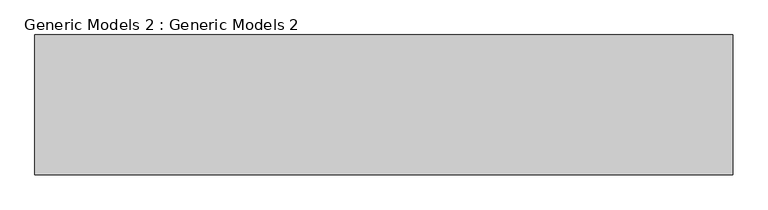
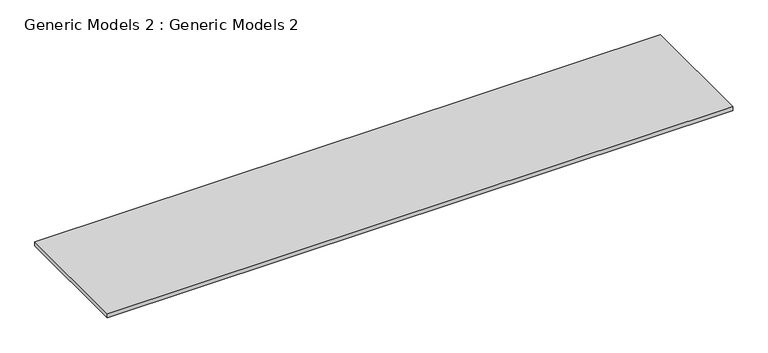
"""IFC4 building model written with IfcOpenShell, lengths in millimetres: proxy geometry, Generic Models 2 : Generic Models 2."""

from ifc_helpers import new_model, si_unit, frame, origin, place, context, project, spatial, polyline, outline, extrude, source, transform, mapped, element, save


def generic_models_2_generic_models_2_f94be15d(model_context):
    return source(origin(), model_context, "Body", "SweptSolid", [
        extrude(outline(polyline([(-10801.6356021, -11016.0591477), (11143.9643979, -11016.0591477), (11143.9643979, -15412.7251081), (-10801.6356021, -15412.7251081), (-10801.6356021, -11016.0591477)])), frame((0.0, 0.0, -152.4), z_axis=(0.0, 0.0, 1.0), x_axis=(1.0, 0.0, 0.0)), (0.0, 0.0, 1.0), 152.4),
    ])


if __name__ == "__main__":
    model = new_model("IFC4")
    model_context = context("Model", 3, world=origin())
    ifc_project = project(units=[si_unit("LENGTHUNIT", "METRE", prefix="MILLI")], contexts=[model_context])
    site = spatial("IfcSite", under=ifc_project)
    building = spatial("IfcBuilding", under=site)
    placement = place(None, origin())
    generic_models_2_generic_models_2_shape = generic_models_2_generic_models_2_f94be15d(model_context)
    element("IfcBuildingElementProxy", 1, Name="Generic Models 2 : Generic Models 2", ObjectType="Generic Models 2 : Generic Models 2", at=placement, inside=building, context=model_context, shape_type="MappedRepresentation", body=[
        mapped(generic_models_2_generic_models_2_shape, transform((0.0, 0.0, 0.0), x_axis=(1.0, 0.0, 0.0), y_axis=(0.0, 1.0, 0.0), z_axis=(0.0, 0.0, 1.0))),
    ])
    save(model, "model.ifc")
